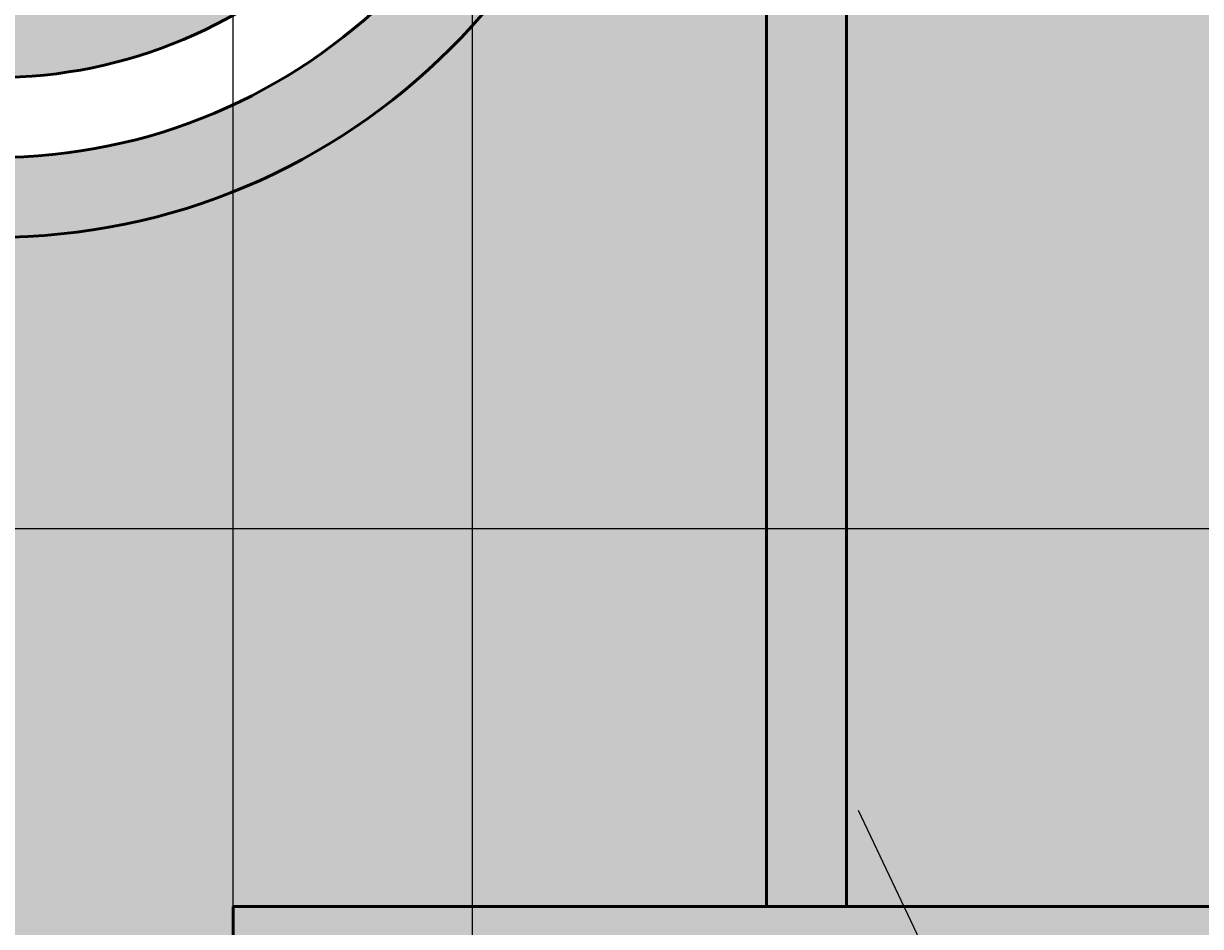
# Model space of a CAD drawing. Units: inches. Extents: x -12 to 334, y -10 to 186.
# Tile 51 of 77: x 227 to 257, y 46 to 69. Entities that reach past the tile are written whole.
import ezdxf
from ezdxf import colors
from ezdxf.entities.mleader import LeaderData, LeaderLine
from ezdxf.math import Vec2, Vec3

# ---------------------------------------------------------------- set-up
doc = ezdxf.new("R2010")
doc.units = ezdxf.units.IN
doc.header["$MEASUREMENT"] = 0
for name, color, linetype, lineweight in [('M-ANNO-TEXT', 3, 'Continuous', 25), ('M-DIMS', 2, 'Continuous', 18), ('M-EQPM', 7, 'Continuous', 50), ('M-EQPM-PATT', 8, 'Continuous', 18)]:
    doc.layers.add(name, color=color, linetype=linetype, lineweight=lineweight)
doc.styles.get("Standard").update_dxf_attribs({"font": 'arial.ttf'})
doc.dimstyles.get("Standard").update_dxf_attribs({"dimtxt": 0.18, "dimasz": 0.18, "dimexe": 0.18, "dimexo": 0.0625, "dimgap": 0.09, "dimtad": 0, "dimtih": 1, "dimtoh": 1, "dimdec": 4, "dimzin": 0, "dimdsep": 46, "dimtxsty": 'Standard', "dimcen": 0.09, "dimadec": 0, "dimazin": 0, "dimtfac": 1, "dimtdec": 4, "dimtofl": 0, "dimtmove": 0, "dimatfit": 3, "dimfxl": 1, "dimtolj": 1, "dimtzin": 0, "dimarcsym": 0})

# ---------------------------------------------------------------- blocks, each defined once
blk = doc.blocks.new('*D1')
at = {"layer": 'Defpoints', "color": 0, "transparency": 16777216}
for p in [(281.426, 91.899), (3.376, 80.692), (281.426, 14.304)]:
    blk.add_point(p, dxfattribs=at)
at = {"layer": 'M-DIMS', "color": 0, "lineweight": -2, "transparency": 16777216}
for p, q in [((281.426, 91.836), (281.426, 14.124)), ((3.376, 80.629), (3.376, 14.124)), ((3.556, 14.304), (141.935, 14.304)), ((281.246, 14.304), (142.867, 14.304))]:
    blk.add_line(p, q, dxfattribs=at)
at = {"layer": 'M-DIMS', "color": 0, "transparency": 16777216}
for points in [[(3.556, 14.334), (3.556, 14.274), (3.376, 14.304)], [(281.246, 14.334), (281.246, 14.274), (281.426, 14.304)]]:
    blk.add_solid(points, dxfattribs=at)
at = {"layer": 'M-DIMS', "color": 0, "transparency": 16777216, "insert": (142.401, 14.304), "char_height": 0.18, "attachment_point": 5}
blk.add_mtext('\\A1;278.05', dxfattribs=at)
blk = doc.blocks.new('*D17')
at = {"layer": 'Defpoints', "color": 0, "transparency": 16777216}
for p in [(106.177, 102.896), (105.892, 56.321), (295.976, 56.321)]:
    blk.add_point(p, dxfattribs=at)
at = {"layer": 'M-DIMS', "color": 0, "lineweight": -2, "transparency": 16777216}
for p, q in [((106.24, 102.896), (296.156, 102.896)), ((295.976, 102.716), (295.976, 79.79)), ((295.976, 56.501), (295.976, 79.426)), ((105.954, 56.321), (296.156, 56.321))]:
    blk.add_line(p, q, dxfattribs=at)
at = {"layer": 'M-DIMS', "color": 0, "transparency": 16777216}
for points in [[(295.946, 102.716), (296.006, 102.716), (295.976, 102.896)], [(295.946, 56.501), (296.006, 56.501), (295.976, 56.321)]]:
    blk.add_solid(points, dxfattribs=at)
at = {"layer": 'M-DIMS', "color": 0, "transparency": 16777216, "insert": (295.976, 79.608), "char_height": 0.18, "attachment_point": 5}
blk.add_mtext('\\A1;46.575', dxfattribs=at)
blk = doc.blocks.new('*D27')
at = {"layer": 'Defpoints', "color": 0, "transparency": 16777216}
for p in [(238.576, 169.385), (216.576, 32.854), (238.576, 32.854)]:
    blk.add_point(p, dxfattribs=at)
at = {"layer": 'M-DIMS', "color": 0, "lineweight": -2, "transparency": 16777216}
for p, q in [((216.576, 32.917), (216.576, 169.565)), ((238.576, 32.917), (238.576, 169.565)), ((216.756, 169.385), (227.357, 169.385)), ((238.396, 169.385), (227.796, 169.385))]:
    blk.add_line(p, q, dxfattribs=at)
at = {"layer": 'M-DIMS', "color": 0, "transparency": 16777216}
for points in [[(216.756, 169.415), (216.756, 169.355), (216.576, 169.385)], [(238.396, 169.415), (238.396, 169.355), (238.576, 169.385)]]:
    blk.add_solid(points, dxfattribs=at)
at = {"layer": 'M-DIMS', "color": 0, "transparency": 16777216, "insert": (227.576, 169.385), "char_height": 0.18, "attachment_point": 5}
blk.add_mtext('\\A1;22', dxfattribs=at)
blk = doc.blocks.new('*D28')
at = {"layer": 'Defpoints', "color": 0, "transparency": 16777216}
for p in [(232.576, 169.385), (222.576, 30.854), (232.576, 30.854)]:
    blk.add_point(p, dxfattribs=at)
at = {"layer": 'M-DIMS', "color": 0, "lineweight": -2, "transparency": 16777216}
for p, q in [((222.576, 30.917), (222.576, 169.565)), ((232.576, 30.917), (232.576, 169.565)), ((222.756, 169.385), (227.366, 169.385)), ((232.396, 169.385), (227.786, 169.385))]:
    blk.add_line(p, q, dxfattribs=at)
at = {"layer": 'M-DIMS', "color": 0, "transparency": 16777216}
for points in [[(222.756, 169.415), (222.756, 169.355), (222.576, 169.385)], [(232.396, 169.415), (232.396, 169.355), (232.576, 169.385)]]:
    blk.add_solid(points, dxfattribs=at)
at = {"layer": 'M-DIMS', "color": 0, "transparency": 16777216, "insert": (227.576, 169.385), "char_height": 0.18, "attachment_point": 5}
blk.add_mtext('\\A1;10', dxfattribs=at)
blk = doc.blocks.new('*D37')
at = {"layer": 'Defpoints', "color": 0, "transparency": 16777216}
for p in [(245.935, 169.385), (232.576, 46.854), (245.935, 46.854)]:
    blk.add_point(p, dxfattribs=at)
at = {"layer": 'M-DIMS', "color": 0, "lineweight": -2, "transparency": 16777216}
for p, q in [((232.576, 46.917), (232.576, 169.565)), ((245.935, 46.917), (245.935, 169.565)), ((232.756, 169.385), (238.871, 169.385)), ((245.755, 169.385), (239.641, 169.385))]:
    blk.add_line(p, q, dxfattribs=at)
at = {"layer": 'M-DIMS', "color": 0, "transparency": 16777216}
for points in [[(232.756, 169.415), (232.756, 169.355), (232.576, 169.385)], [(245.755, 169.415), (245.755, 169.355), (245.935, 169.385)]]:
    blk.add_solid(points, dxfattribs=at)
at = {"layer": 'M-DIMS', "color": 0, "transparency": 16777216, "insert": (239.256, 169.385), "char_height": 0.18, "attachment_point": 5}
blk.add_mtext('\\A1;13.36', dxfattribs=at)
blk = doc.blocks.new('*D38')
at = {"layer": 'Defpoints', "color": 0, "transparency": 16777216}
for p in [(247.935, 82.697), (247.935, 46.854), (295.976, 46.854)]:
    blk.add_point(p, dxfattribs=at)
at = {"layer": 'M-DIMS', "color": 0, "lineweight": -2, "transparency": 16777216}
for p, q in [((247.998, 82.697), (296.156, 82.697)), ((295.976, 82.517), (295.976, 64.957)), ((295.976, 47.034), (295.976, 64.594)), ((247.998, 46.854), (296.156, 46.854))]:
    blk.add_line(p, q, dxfattribs=at)
at = {"layer": 'M-DIMS', "color": 0, "transparency": 16777216}
for points in [[(295.946, 82.517), (296.006, 82.517), (295.976, 82.697)], [(295.946, 47.034), (296.006, 47.034), (295.976, 46.854)]]:
    blk.add_solid(points, dxfattribs=at)
at = {"layer": 'M-DIMS', "color": 0, "transparency": 16777216, "insert": (295.976, 64.775), "char_height": 0.18, "attachment_point": 5}
blk.add_mtext('\\A1;35.84', dxfattribs=at)
blk = doc.blocks.new('*D39')
at = {"layer": 'Defpoints', "color": 0, "transparency": 16777216}
for p in [(279.726, 80.692), (-11.174, 45.854), (269.381, 45.854)]:
    blk.add_point(p, dxfattribs=at)
at = {"layer": 'M-DIMS', "color": 0, "lineweight": -2, "transparency": 16777216}
for p, q in [((279.664, 80.692), (-11.354, 80.692)), ((-11.174, 80.512), (-11.174, 63.455)), ((-11.174, 46.034), (-11.174, 63.091)), ((269.318, 45.854), (-11.354, 45.854))]:
    blk.add_line(p, q, dxfattribs=at)
at = {"layer": 'M-DIMS', "color": 0, "transparency": 16777216}
for points in [[(-11.204, 80.512), (-11.144, 80.512), (-11.174, 80.692)], [(-11.204, 46.034), (-11.144, 46.034), (-11.174, 45.854)]]:
    blk.add_solid(points, dxfattribs=at)
at = {"layer": 'M-DIMS', "color": 0, "transparency": 16777216, "insert": (-11.174, 63.273), "char_height": 0.18, "attachment_point": 5}
blk.add_mtext('\\A1;34.84', dxfattribs=at)
blk = doc.blocks.new('*D41')
at = {"layer": 'Defpoints', "color": 0, "transparency": 16777216}
for p in [(190.169, 91.899), (277.343, 68.515)]:
    blk.add_point(p, dxfattribs=at)
at = {"layer": 'M-DIMS', "color": 0, "lineweight": -2, "transparency": 16777216}
for p, q in [((190.169, 91.809), (190.169, 91.989)), ((190.079, 91.899), (190.259, 91.899)), ((329.648, 54.485), (277.517, 68.469)), ((329.828, 54.485), (329.648, 54.485))]:
    blk.add_line(p, q, dxfattribs=at)
at = {"layer": 'M-DIMS', "color": 0, "transparency": 16777216}
blk.add_solid([(277.525, 68.498), (277.509, 68.44), (277.343, 68.515)], dxfattribs=at)
at = {"layer": 'M-DIMS', "color": 0, "transparency": 16777216, "insert": (330.307, 54.485), "char_height": 0.18, "attachment_point": 5}
blk.add_mtext('\\A1;R90.26', dxfattribs=at)

msp = doc.modelspace()

# ---------------------------------------------------------------- hatches: boundary and pattern name
at = {"layer": 'M-EQPM-PATT'}
h = msp.add_hatch(color=256, dxfattribs=at)
h.set_gradient(color1=(99, 100, 102), color2=(99, 100, 102), tint=1)
h.paths.add_polyline_path([(126.9567, 136.8871), (179.7818, 136.8871), (180.0106, 137.8871), (126.3793, 137.8871), (106.1771, 102.8958), (86.8879, 102.8958), (86.8879, 109.0583), (84.7229, 109.0583), (84.7229, 100.8958), (106.1771, 100.8958)])
h.paths.add_polyline_path([(196.3421, 152.8345), (195.3421, 152.8345), (195.3421, 137.8871), (180.0106, 137.8871), (179.7818, 136.8871), (196.3421, 136.8871)])
h.paths.add_polyline_path([(215.0166, 152.8345), (214.0166, 152.8345), (214.0166, 136.9435), (268.3808, 136.9435, -0.2673785), (268.3808, 46.8541), (249.3759, 46.8541), (249.8485, 45.8541), (269.3808, 45.8541, 0.2615891), (269.3808, 137.9435), (215.0166, 137.9435)])
h = msp.add_hatch(color=256, dxfattribs=at)
h.set_gradient(color1=(99, 100, 102), color2=(99, 100, 102), tint=1)
h.paths.add_polyline_path([(4.3766, 80.754, -0.4132606), (23.5807, 99.8958), (37.1002, 99.8958), (37.1002, 127.7078), (32.1002, 127.7078), (32.1002, 125.2078), (36.1002, 125.2078), (36.1002, 100.8958), (23.5807, 100.8958, 1), (23.5807, 60.4872), (36.1002, 60.4872), (36.1002, 36.1752), (32.1002, 36.1752), (32.1002, 33.6752), (37.1002, 33.6752), (37.1002, 61.4872), (23.5807, 61.4872, -0.384914), (4.4744, 78.754), (72.9244, 78.754), (72.9244, 69.6117), (75.9244, 69.6117), (75.9244, 89.8963), (72.9244, 89.8963), (72.9244, 80.754)])
h.paths.add_polyline_path([(54.1002, 125.2078), (58.1002, 125.2078), (58.1002, 127.7078), (53.1002, 127.7078), (53.1002, 99.8958), (64.5, 99.8958), (64.5, 109.0583), (63.5, 109.0583), (63.5, 100.8958), (54.1002, 100.8958)], flags=17)
h.paths.add_polyline_path([(53.1002, 33.6752), (58.1002, 33.6752), (58.1002, 36.1752), (54.1002, 36.1752), (54.1002, 60.4872), (64.2068, 60.4872), (64.2068, 49.4497), (87.8879, 49.4497), (87.8879, 55.3205), (104.8919, 55.3205), (104.8919, 30.8541), (99.8919, 30.8541), (99.8919, 28.8541), (105.8919, 28.8541), (105.8919, 56.3205), (87.8879, 56.3205), (87.8879, 63.6117), (86.8879, 63.6117), (86.8879, 50.4497), (65.0061, 50.4497), (65.0061, 63.6117), (64.5, 63.6117), (64.5, 61.4872), (53.1002, 61.4872)])
h.paths.add_polyline_path([(121.8919, 28.8541), (121.8919, 30.8541), (116.8919, 30.8541), (116.8919, 45.8541), (209.6965, 45.8541), (209.9204, 46.8541), (115.8919, 46.8541), (115.8919, 28.8541)])
h.paths.add_polyline_path([(221.5761, 32.8541), (216.5761, 32.8541), (216.5761, 30.8541), (222.5761, 30.8541), (222.5761, 46.8541), (209.9204, 46.8541), (209.6965, 45.8541), (221.5761, 45.8541)])
h.paths.add_polyline_path([(233.5761, 45.8541), (249.8485, 45.8541), (249.3759, 46.8541), (232.5761, 46.8541), (232.5761, 30.8541), (238.5761, 30.8541), (238.5761, 32.8541), (233.5761, 32.8541)])
h = msp.add_hatch(color=256, dxfattribs=at)
h.set_gradient(color1=(205, 32, 39), color2=(205, 32, 39), tint=1)
h.paths.add_polyline_path([(64.5, 80.754), (64.5, 89.8963), (226.6083, 89.8963, -1), (226.6083, 69.6117), (64.5, 69.6117), (64.5, 78.754), (4.4744, 78.754, 0.384914), (23.5807, 61.4872), (37.1002, 61.4872), (37.1002, 33.6752), (53.1002, 33.6752), (53.1002, 61.4872), (64.5, 61.4872), (64.5, 63.6117), (226.6083, 63.6117, 1), (226.6083, 95.8963), (64.5, 95.8963), (64.5, 99.8958), (53.1002, 99.8958), (53.1002, 127.7078), (37.1002, 127.7078), (37.1002, 99.8958), (23.5807, 99.8958, 0.4132606), (4.3766, 80.754)])
h.paths.add_polyline_path([(64.5, 91.8963), (64.5, 93.8963), (226.6083, 93.8963, -1), (226.6083, 65.6117), (64.5, 65.6117), (64.5, 67.6117), (226.6083, 67.6117, 1), (226.6083, 91.8963)], flags=16)
h = msp.add_hatch(color=256, dxfattribs=at)
h.set_gradient(color1=(94, 103, 175), color2=(94, 103, 175), tint=1)
h.paths.add_polyline_path([(129.093, 89.8963), (86.8879, 89.8963), (86.8879, 69.6117), (129.093, 69.6117)], flags=17)
h.paths.add_polyline_path([(170.9079, 89.8963), (130.8573, 89.8963), (130.8573, 69.6117), (170.9079, 69.6117)], flags=17)
h.paths.add_polyline_path([(216.4278, 89.8963), (172.6722, 89.8963), (172.6722, 69.6117), (216.4278, 69.6117)], flags=17)
h.paths.add_polyline_path([(245.9354, 82.6969), (247.9354, 82.6969), (247.9354, 46.8541), (268.3808, 46.8541, 0.0998398), (279.7263, 80.6915), (251.9801, 80.6915, 0.4142136), (231.7758, 100.8958), (84.7229, 100.8958), (84.7229, 109.0583), (83.7229, 109.0583), (83.7229, 95.8963), (129.093, 95.8963), (129.093, 98.1081), (130.8573, 98.1081), (130.8573, 95.8963), (170.9079, 95.8963), (170.9079, 98.1081), (172.6722, 98.1081), (172.6722, 95.8963), (216.4278, 95.8963), (216.4278, 98.1081), (218.1922, 98.1081), (218.1922, 95.8963), (226.6083, 95.8963, -1), (226.6083, 63.6117), (218.1922, 63.6117), (218.1922, 61.1045), (216.4278, 61.1045), (216.4278, 63.6117), (172.6722, 63.6117), (172.6722, 61.1045), (170.9079, 61.1045), (170.9079, 63.6117), (130.8573, 63.6117), (130.8573, 61.1045), (129.093, 61.1045), (129.093, 63.6117), (87.8879, 63.6117), (87.8879, 56.3205), (105.8919, 56.3205), (105.8919, 28.8541), (115.8919, 28.8541), (115.8919, 46.8541), (222.5761, 46.8541), (222.5761, 30.8541), (232.5761, 30.8541), (232.5761, 46.8541), (245.9354, 46.8541)])
h.paths.add_polyline_path([(86.8879, 89.8963), (75.9244, 89.8963), (75.9244, 69.6117), (86.8879, 69.6117)])
h.paths.add_polyline_path([(83.7229, 109.0583), (75.9244, 109.0583), (75.9244, 95.8963), (83.7229, 95.8963)])
h.paths.add_polyline_path([(226.6083, 89.8963), (218.1922, 89.8963), (218.1922, 69.6117), (226.6083, 69.6117, 1)], flags=17)
h = msp.add_hatch(color=256, dxfattribs=at)
h.set_gradient(color1=(0, 0, 255), color2=(0, 0, 255), tint=1)
h.paths.add_polyline_path([(84.7229, 100.8958), (84.7229, 109.0583), (83.7229, 109.0583), (83.7229, 95.8963), (129.093, 95.8963), (129.093, 98.1081), (130.8573, 98.1081), (130.8573, 95.8963), (170.9079, 95.8963), (170.9079, 98.1081), (172.6722, 98.1081), (172.6722, 95.8963), (216.4278, 95.8963), (216.4278, 98.1081), (218.1922, 98.1081), (218.1922, 95.8963), (226.6083, 95.8963, -1), (226.6083, 63.6117), (218.1922, 63.6117), (218.1922, 61.1045), (216.4278, 61.1045), (216.4278, 63.6117), (172.6722, 63.6117), (172.6722, 61.1045), (170.9079, 61.1045), (170.9079, 63.6117), (130.8573, 63.6117), (130.8573, 61.1045), (129.093, 61.1045), (129.093, 63.6117), (87.8879, 63.6117), (87.8879, 56.3205), (105.8919, 56.3205), (105.8919, 28.8541), (115.8919, 28.8541), (115.8919, 46.8541), (222.5761, 46.8541), (222.5761, 30.8541), (232.5761, 30.8541), (232.5761, 46.8541), (245.9354, 46.8541), (245.9354, 82.6969), (247.9354, 82.6969), (247.9354, 46.8541), (268.3808, 46.8541, 0.0998398), (279.7263, 80.6915), (251.9801, 80.6915, 0.4142136), (231.7758, 100.8958)])
h = msp.add_hatch(color=256, dxfattribs=at)
h.set_gradient(color1=(241, 235, 31), color2=(244, 238, 81), tint=1)
h.paths.add_polyline_path([(245.9354, 46.8541), (247.9354, 46.8541), (247.9354, 82.6969), (245.9354, 82.6969)])

# ---------------------------------------------------------------- linework, layer by layer
at = {"layer": 'M-EQPM'}
for p, q in [((245.9354, 82.6969), (245.9354, 46.8541)), ((247.9354, 82.6969), (247.9354, 46.8541)), ((268.3808, 46.8541), (232.5761, 46.8541)), ((232.5761, 46.8541), (232.5761, 30.8541))]:
    msp.add_line(p, q, dxfattribs=at)
for points in [[(64.5, 63.6117), (226.6083, 63.6117, 1), (226.6083, 95.8963), (64.5, 95.8963)], [(64.5, 65.6117), (226.6083, 65.6117, 1), (226.6083, 93.8963), (64.5, 93.8963)], [(64.5, 67.6117), (226.6083, 67.6117, 1), (226.6083, 91.8963), (64.5, 91.8963)]]:
    msp.add_lwpolyline(points, format="xyb", dxfattribs=at)

# ---------------------------------------------------------------- dimensions: what is measured, and where the dimension line sits
at = {"layer": 'M-DIMS'}
for base, p1, p2, override, picture, middle in [((238.5761, 169.3845), (216.5761, 32.8541), (238.5761, 32.8541), {"dimdec": 0, "dimlfac": 1, "dimrnd": 0, "dimzin": 0, "dimdsep": 46, "dimlunit": 2}, '*D27', (227.5761, 169.3845)), ((232.5761, 169.3845), (222.5761, 30.8541), (232.5761, 30.8541), {"dimdec": 0, "dimlfac": 1, "dimrnd": 0, "dimzin": 0, "dimdsep": 46, "dimlunit": 2}, '*D28', (227.5761, 169.3845)), ((245.9354, 169.3845), (232.5761, 46.8541), (245.9354, 46.8541), {"dimdec": 2, "dimlfac": 1, "dimrnd": 0, "dimzin": 0, "dimdsep": 46, "dimlunit": 2}, '*D37', (239.2558, 169.3845)), ((281.4256, 14.3041), (3.3765, 80.6915), (281.4256, 91.8988), {"dimdec": 2, "dimlfac": 1, "dimrnd": 0, "dimzin": 0, "dimdsep": 46, "dimlunit": 2}, '*D1', (142.401, 14.3041))]:
    dim = msp.add_linear_dim(base=base, p1=p1, p2=p2, dimstyle='Standard', override=override, dxfattribs=at)
    dim.commit()
    dim.dimension.update_dxf_attribs({"geometry": picture, "text_midpoint": middle})
for base, p1, p2, override, picture, middle in [((295.9756, 56.3205), (106.1771, 102.8958), (105.8919, 56.3205), {"dimdec": 3, "dimlfac": 1, "dimrnd": 0, "dimzin": 0, "dimdsep": 46, "dimlunit": 2}, '*D17', (295.9756, 79.6082)), ((295.9756, 46.8541), (247.9354, 82.6969), (247.9354, 46.8541), {"dimdec": 2, "dimlfac": 1, "dimrnd": 0, "dimzin": 0, "dimdsep": 46, "dimlunit": 2}, '*D38', (295.9756, 64.7755)), ((-11.1736, 45.8541), (279.7263, 80.6915), (269.3808, 45.8541), {"dimdec": 2, "dimlfac": 1, "dimrnd": 0, "dimzin": 0, "dimdsep": 46, "dimlunit": 2}, '*D39', (-11.1735, 63.2728))]:
    dim = msp.add_linear_dim(base=base, p1=p1, p2=p2, angle=90, dimstyle='Standard', override=override, dxfattribs=at)
    dim.commit()
    dim.dimension.update_dxf_attribs({"geometry": picture, "text_midpoint": middle})
dim = msp.add_radius_dim(center=(190.1689, 91.8988), mpoint=(277.3431, 68.5153), dimstyle='Standard', override={"dimdec": 2, "dimlfac": 1, "dimrnd": 0, "dimzin": 0, "dimdsep": 46, "dimlunit": 2}, dxfattribs=at)
dim.commit()
dim.dimension.update_dxf_attribs({"geometry": '*D41', "text_midpoint": (330.3074, 54.4851), "dimtype": 164})

# ---------------------------------------------------------------- leaders
at = {"layer": 'M-ANNO-TEXT'}
ml = msp.add_multileader_mtext('Standard', dxfattribs=at)
ml.set_content('^I^IWeir', color=256)
ml.set_leader_properties()
ml.build(insert=Vec2(0, 0))
ml.multileader.update_dxf_attribs({"dogleg_length": 0.36, "arrow_head_size": 0.7})
ctx = ml.context
ctx.base_point, ctx.arrow_head_size, ctx.landing_gap_size, ctx.plane_origin = Vec3(257.1525, 34.1955), 0.7, 0.09, Vec3(247.9354, 49.9015)
notes = []
notes.append((ctx, [(0, (1, 1, 0), (255.3593, 34.1955), (1, 0), 1.7932, [(0, [(247.9354, 49.9015)], 0, [])])]))
ctx.mtext.insert, ctx.mtext.flow_direction = Vec3(257.2425, 36.2283), 5
for ctx, leaders in notes:
    for number, flags, end, landing, length, lines in leaders:
        leader = LeaderData()
        leader.index, (leader.has_last_leader_line, leader.has_dogleg_vector, leader.attachment_direction) = number, flags
        leader.last_leader_point, leader.dogleg_vector, leader.dogleg_length = Vec3(end), Vec3(landing), length
        for number, points, colour, breaks in lines:
            line = LeaderLine()
            line.index, line.vertices, line.color, line.breaks = number, Vec3.list(points), colors.encode_raw_color(colour), breaks
            leader.lines.append(line)
        ctx.leaders.append(leader)

doc.saveas('drawing.dxf')
